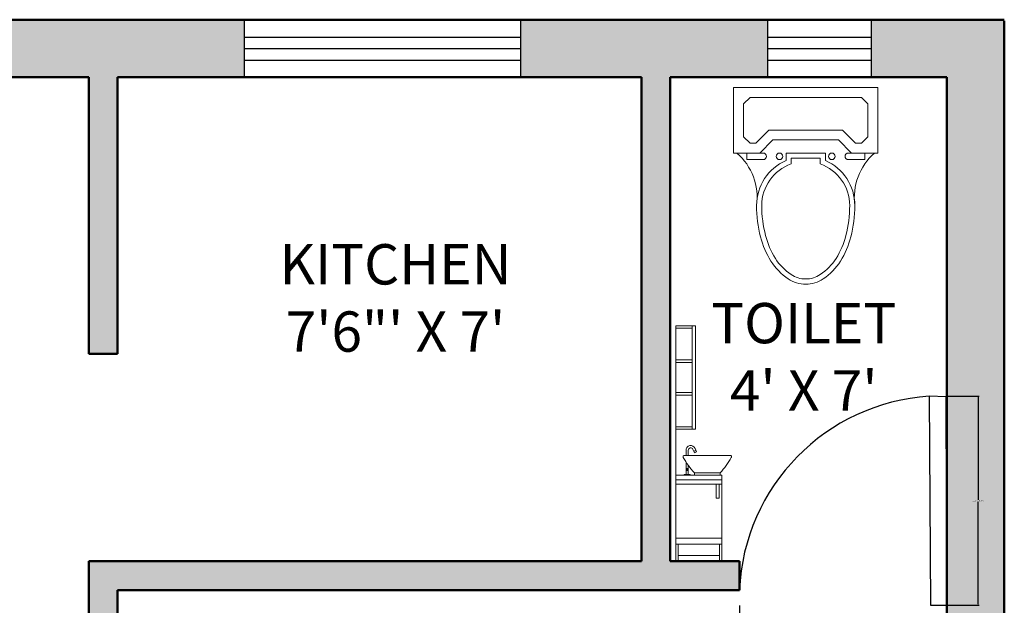
# Model space of a CAD drawing. Units: inches. Extents: x 1771 to 3025, y 319 to 889.
# Tile 35 of 35: x 2854 to 3025, y 788 to 889. Entities that reach past the tile are written whole.
import ezdxf

# ---------------------------------------------------------------- set-up
doc = ezdxf.new("R2010")
doc.units = ezdxf.units.IN
doc.header["$MEASUREMENT"] = 0
for name, color, linetype, lineweight in [('A-ANNO-DIMS', 2, 'Continuous', 18), ('A-AREA-IDEN', 241, 'Continuous', 25), ('A-DOOR', 4, 'Continuous', 25), ('A-FLOR-FIXT', 8, 'Continuous', 18), ('A-GLAZ', 40, 'Continuous', 25), ('A-WALL', 7, 'Continuous', 50), ('A-WALL-PATT', 254, 'Continuous', 13)]:
    doc.layers.add(name, color=color, linetype=linetype, lineweight=lineweight)
doc.styles.get("Standard").update_dxf_attribs({"font": 'arial.ttf'})
doc.dimstyles.get("Standard").update_dxf_attribs({"dimtxt": 0.18, "dimasz": 0.18, "dimexe": 0.18, "dimexo": 0.0625, "dimgap": 0.09, "dimtad": 0, "dimtih": 1, "dimtoh": 1, "dimdec": 4, "dimzin": 0, "dimdsep": 46, "dimtxsty": 'Standard', "dimcen": 0.09, "dimadec": 0, "dimazin": 0, "dimtfac": 1, "dimtdec": 4, "dimtofl": 0, "dimtmove": 0, "dimatfit": 3, "dimfxl": 1, "dimtolj": 1, "dimtzin": 0, "dimarcsym": 0})

# ---------------------------------------------------------------- blocks, each defined once
blk = doc.blocks.new('A$C098B081F')
for p, q in [((558.8, 762), (0, 762)), ((0, 762), (0, 508)), ((558.8, 762), (558.8, 508)), ((63.5, 723.9), (38.1, 698.5)), ((38.1, 698.5), (38.1, 571.5)), ((495.3, 723.9), (63.5, 723.9)), ((520.7, 698.5), (495.3, 723.9)), ((520.7, 698.5), (520.7, 571.5)), ((136.6, 596.9), (85.8, 546.1)), ((422.2, 596.9), (136.6, 596.9)), ((422.2, 596.9), (473, 546.1)), ((38.1, 571.5), (63.5, 546.1)), ((63.5, 546.1), (85.8, 546.1)), ((152.4, 558.8), (101.6, 508)), ((406.4, 558.8), (152.4, 558.8)), ((406.4, 558.8), (457.2, 508)), ((495.3, 546.1), (473, 546.1)), ((495.3, 546.1), (520.7, 571.5)), ((0, 508), (12.7, 508)), ((12.7, 508), (101.6, 508)), ((50.8, 508), (50.8, 482.6)), ((50.8, 508), (101.6, 508)), ((114.3, 508), (101.6, 508)), ((203.2, 508), (203.2, 479.4)), ((203.2, 508), (355.6, 508)), ((355.6, 508), (355.6, 479.4)), ((444.5, 508), (457.2, 508)), ((508, 508), (457.2, 508)), ((508, 508), (546.1, 508)), ((508, 508), (508, 482.6)), ((558.8, 508), (546.1, 508)), ((50.8, 482.6), (114.3, 482.6)), ((223.2, 488), (223.2, 465.8)), ((223.2, 488), (335.6, 488)), ((335.6, 488), (335.6, 465.8)), ((508, 482.6), (444.5, 482.6))]:
    blk.add_line(p, q)
for centre in [(177.8, 495.3), (381, 495.3)]:
    blk.add_circle(centre, 12.7)
for centre, radius, start, end in [((-137.5, 335.8), 228.5, 352.2011, 48.911), ((114.3, 495.3), 12.7, 270, 90), ((444.5, 495.3), 12.7, 90, 270), ((696.3, 335.8), 228.5, 131.089, 187.7989), ((279.4, 304.8), 190.5, 113.5782, 180), ((279.4, 304.8), 170.5, 109.2456, 180), ((279.4, 304.8), 170.5, 0, 70.7544), ((279.4, 304.8), 190.5, 0, 66.4218), ((574.9, 304.8), 486, 180, 194.5143), ((574.9, 304.8), 466, 180, 194.5143), ((-16.1, 304.8), 466, 345.4857, 360), ((-16.1, 304.8), 486, 345.4857, 360), ((429.2, 267.1), 335.5, 194.5143, 212.0054), ((429.2, 267.1), 315.5, 194.5143, 212.0054), ((129.6, 267.1), 315.5, 327.9946, 345.4857), ((129.6, 267.1), 335.5, 327.9946, 345.4857), ((337.2, 209.6), 227, 212.0054, 236.4659), ((337.2, 209.6), 207, 212.0054, 236.4659), ((221.6, 209.6), 207, 303.5341, 327.9946), ((221.6, 209.6), 227, 303.5341, 327.9946), ((279.4, 122.4), 122.4, 236.4659, 270), ((279.4, 122.4), 102.4, 236.4659, 270), ((279.4, 122.4), 102.4, 270, 303.5341), ((279.4, 122.4), 122.4, 270, 303.5341)]:
    blk.add_arc(centre, radius, start, end)
blk = doc.blocks.new('A$C3EAC730C')
for p, q in [((0, 2.05), (0.17, 2.05)), ((0, 2.05), (0, 0.2)), ((0, 2.03), (0.14, 2.03)), ((0.14, 2.05), (0.14, 1.15)), ((0.17, 2.05), (0.17, 1.15)), ((0, 1.7542), (0.14, 1.7542)), ((0, 1.7292), (0.14, 1.7292)), ((0, 1.4708), (0.14, 1.4708)), ((0, 1.4458), (0.14, 1.4458)), ((0, 1.17), (0.14, 1.17)), ((0, 1.15), (0.17, 1.15)), ((0.0877, 0.964), (0.0877, 0.92)), ((0.1077, 0.9647), (0.1077, 0.92)), ((0.1601, 0.9446), (0.1481, 0.9744)), ((0.1545, 0.9582), (0.1731, 0.9657)), ((0.1552, 0.9563), (0.1739, 0.9639)), ((0.1601, 0.9446), (0.1787, 0.9521)), ((0.1787, 0.9521), (0.1666, 0.9819)), ((0.0627, 0.915), (0.0627, 0.9063)), ((0.0677, 0.92), (0.4777, 0.92)), ((0.0877, 0.8637), (0.0877, 0.756)), ((0.4827, 0.915), (0.4827, 0.9063)), ((0.4827, 0.915), (0.4827, 0.9063)), ((0.0902, 0.7905), (0.1052, 0.7905)), ((0.0902, 0.7905), (0.0902, 0.756)), ((0.0947, 0.8022), (0.0947, 0.7905)), ((0.1007, 0.8022), (0.1007, 0.7905)), ((0.1052, 0.7905), (0.1052, 0.756)), ((0.1077, 0.8346), (0.1077, 0.756)), ((0.4, 0.75), (0, 0.75)), ((0.4, 0.71), (0, 0.71)), ((0.0577, 0.75), (0.1037, 0.75)), ((0.0727, 0.756), (0.0727, 0.75)), ((0.1227, 0.756), (0.0727, 0.756)), ((0.1227, 0.756), (0.1227, 0.75)), ((0.1602, 0.77), (0.1602, 0.75)), ((0.1602, 0.77), (0.3852, 0.77)), ((0.1602, 0.75), (0.3852, 0.75)), ((0.3852, 0.77), (0.3852, 0.75)), ((0.4, 0.71), (0.4, 0.75)), ((0.4, 0.72), (0.4, 0.2)), ((0.4, 0.67), (0, 0.67)), ((0.35, 0.55), (0.35, 0.67)), ((0.375, 0.55), (0.375, 0.67)), ((0.35, 0.55), (0.375, 0.55)), ((0.4, 0.2), (0, 0.2)), ((0, 0.2), (0, 0)), ((0.4, 0), (0.4, 0.2)), ((0.4, 0.15), (0, 0.15)), ((0.02, 0.15), (0.02, 0)), ((0.38, 0), (0.38, 0.15)), ((0, 0), (0.4, 0)), ((0.02, 0.05), (0.38, 0.05))]:
    blk.add_line(p, q)
blk.add_circle((0.0977, 0.804), 0.0035)
for centre, radius, start, end in [((0.1286, 0.9665), 0.041, 22.01327, 183.41193), ((0.1286, 0.9665), 0.021, 22.01327, 184.76808), ((0.0677, 0.915), 0.005, 90, 180), ((0.0677, 0.9063), 0.005, 180, 209.45502), ((0.7052, 1.2664), 0.7372, 209.45502, 222.32259), ((-0.1599, 1.2664), 0.7372, 317.67741, 330.54498), ((0.4777, 0.915), 0.005, 0, 90), ((0.4777, 0.9063), 0.005, 330.54498, 0)]:
    blk.add_arc(centre, radius, start, end)
blk = doc.blocks.new('DOOR-35')
blk.add_lwpolyline([(35.88, 36.19), (32.96, 36.3), (33.16, 0), (36, 0.05)], close=True)
blk.add_arc((35.23, 1.11), 35.26, 93.6879, 177.4925)
blk = doc.blocks.new('WIN-48')
for p, q in [((0, 0), (0, 10)), ((48, 0), (48, 10)), ((0, 7), (48, 7)), ((0, 5), (48, 5)), ((0, 3), (48, 3))]:
    blk.add_line(p, q)
blk = doc.blocks.new('WIN-18')
for p, q in [((0, 0), (0, 10)), ((18, 0), (18, 10)), ((0, 7), (18, 7)), ((0, 5), (18, 5)), ((0, 3), (18, 3))]:
    blk.add_line(p, q)
blk = doc.blocks.new('*D30')
at = {"layer": 'A-ANNO-DIMS', "color": 0, "lineweight": -2, "transparency": 16777216}
for p, q in [((3014.75, 824.13), (3020.31, 824.13)), ((3020.13, 823.95), (3020.13, 806.16)), ((3020.13, 788.01), (3020.13, 805.8)), ((3014.75, 787.83), (3020.31, 787.83))]:
    blk.add_line(p, q, dxfattribs=at)
at = {"layer": 'A-ANNO-DIMS', "color": 0, "transparency": 16777216}
for points in [[(3020.1, 823.95), (3020.16, 823.95), (3020.13, 824.13)], [(3020.1, 788.01), (3020.16, 788.01), (3020.13, 787.83)]]:
    blk.add_solid(points, dxfattribs=at)
at = {"layer": 'Defpoints', "color": 0, "transparency": 16777216}
for p in [(3014.68, 824.13), (3020.13, 824.13), (3014.68, 787.83)]:
    blk.add_point(p, dxfattribs=at)
at = {"layer": 'A-ANNO-DIMS', "color": 0, "transparency": 16777216, "insert": (3020.13, 805.98), "char_height": 0.18, "attachment_point": 5}
blk.add_mtext('\\A1;DOOR D2 36 TYP.', dxfattribs=at)
blk = doc.blocks.new('*D31')
at = {"layer": 'A-ANNO-DIMS', "color": 0, "lineweight": -2, "transparency": 16777216}
for p, q in [((2978.68, 787.77), (2978.68, 782.21)), ((3014.68, 787.77), (3014.68, 782.21)), ((2978.86, 782.39), (2996.16, 782.39)), ((3014.5, 782.39), (2997.21, 782.39))]:
    blk.add_line(p, q, dxfattribs=at)
at = {"layer": 'A-ANNO-DIMS', "color": 0, "transparency": 16777216}
for points in [[(2978.86, 782.42), (2978.86, 782.36), (2978.68, 782.39)], [(3014.5, 782.42), (3014.5, 782.36), (3014.68, 782.39)]]:
    blk.add_solid(points, dxfattribs=at)
at = {"layer": 'Defpoints', "color": 0, "transparency": 16777216}
for p in [(2978.68, 787.83), (3014.68, 787.83), (3014.68, 782.39)]:
    blk.add_point(p, dxfattribs=at)
at = {"layer": 'A-ANNO-DIMS', "color": 0, "transparency": 16777216, "insert": (2996.68, 782.39), "char_height": 0.18, "attachment_point": 5}
blk.add_mtext('\\A1;36 TYP.', dxfattribs=at)

msp = doc.modelspace()

# ---------------------------------------------------------------- hatches: boundary and pattern name
at = {"layer": 'A-WALL-PATT'}
h = msp.add_hatch(color=256, dxfattribs=at)
h.dxf.hatch_style = 1
h.paths.add_polyline_path([(2870.68, 879.48), (2892.73, 879.48), (2892.73, 889.48), (2842.68, 889.48), (2842.68, 879.48), (2865.68, 879.48), (2865.68, 831.48), (2870.68, 831.48)])
h.paths.add_polyline_path([(2983.64, 889.48), (2940.73, 889.48), (2940.73, 879.48), (2961.68, 879.48), (2961.68, 795.48), (2865.68, 795.48), (2865.68, 759.48), (2865.68, 665.48), (2870.68, 665.48), (2870.68, 712.85), (2870.68, 790.48), (2978.68, 790.48), (2978.68, 795.48), (2966.68, 795.48), (2966.68, 879.48), (2983.64, 879.48)])
h.paths.add_polyline_path([(3024.68, 889.48), (3001.64, 889.48), (3001.64, 879.48), (3014.68, 879.48), (3014.68, 790.48), (3014.68, 769.46), (3024.68, 769.46)])
h.paths.add_polyline_path([(3024.68, 721.46), (3014.68, 721.46), (3014.68, 670.48), (2906.68, 670.48), (2906.68, 665.48), (2925.68, 665.48), (2925.68, 653.48), (2930.68, 653.48), (2930.68, 665.48), (3014.68, 665.48), (3014.68, 650.02), (3024.68, 650.02)])
h.paths.add_polyline_path([(3024.68, 632.02), (3014.68, 632.02), (3014.68, 617.48), (2925.68, 617.48), (2906.68, 617.48), (2906.68, 612.48), (3014.68, 612.48), (3014.68, 581.96), (3024.68, 581.96)])
h.paths.add_polyline_path([(3024.68, 533.96), (3014.68, 533.96), (3014.68, 480.48), (2870.68, 480.48), (2870.68, 617.48), (2860.68, 617.48), (2860.68, 544.48), (2769.68, 544.48), (2769.68, 534.48), (2860.68, 534.48), (2860.68, 470.48), (3014.68, 470.48), (3014.68, 453.61), (3024.68, 453.61)])
h.paths.add_polyline_path([(3024.68, 405.61), (3014.68, 405.61), (3014.68, 394.48), (2860.68, 394.48), (2860.68, 384.48), (3024.68, 384.48)])
h.paths.add_polyline_path([(2733.68, 643.43), (2723.68, 643.43), (2723.68, 534.48), (2733.68, 534.48)])
h.paths.add_polyline_path([(2733.68, 754.48), (2829.68, 754.48), (2829.68, 759.48), (2733.68, 759.48), (2733.68, 843.44, -0.008336), (2732.38, 843.48), (2723.68, 843.48), (2723.68, 691.43), (2733.68, 691.43)])
h.paths.add_polyline_path([(2794.68, 889.48), (2723.68, 889.48), (2723.68, 879.48), (2794.68, 879.48)])

# ---------------------------------------------------------------- linework, layer by layer
at = {"layer": 'A-WALL'}
for p, q in [((3024.68, 889.48), (2682.68, 889.48)), ((3024.68, 384.48), (3024.68, 889.28)), ((2865.68, 879.48), (2687.68, 879.48)), ((2865.68, 879.48), (2865.68, 831.48)), ((2961.68, 879.48), (2870.68, 879.48)), ((2870.68, 879.48), (2870.68, 831.48)), ((2961.68, 795.48), (2961.68, 879.48)), ((2966.68, 795.48), (2966.68, 879.48)), ((3014.68, 879.48), (2966.68, 879.48)), ((3014.68, 790.48), (3014.68, 879.48)), ((2870.68, 831.48), (2865.68, 831.48)), ((2961.68, 795.48), (2865.68, 795.48)), ((2865.68, 795.48), (2865.68, 759.48)), ((2978.68, 795.48), (2966.68, 795.48)), ((2978.68, 790.48), (2978.68, 795.48)), ((2978.68, 790.48), (2870.68, 790.48)), ((2870.68, 790.48), (2870.68, 670.48)), ((3014.68, 670.48), (3014.68, 790.48))]:
    msp.add_line(p, q, dxfattribs=at)

# ---------------------------------------------------------------- block references
at = {"layer": 'A-DOOR'}
msp.add_blockref('DOOR-35', (2978.68, 787.83), dxfattribs=at)
at = {"layer": 'A-FLOR-FIXT'}
for name, p, xscale, yscale, zscale in [('A$C098B081F', (2977.68, 843.58), 0.0447923195545138, 0.0447923195545138, 0.0447923195545138), ('A$C3EAC730C', (2967.66, 795.48), 19.93356852258053, 19.93356852258053, 19.93356852258053)]:
    msp.add_blockref(name, p, dxfattribs=dict(at, xscale=xscale, yscale=yscale, zscale=zscale))
at = {"layer": 'A-GLAZ'}
for name, p in [('WIN-48', (2892.73, 879.48)), ('WIN-18', (2983.64, 879.48))]:
    msp.add_blockref(name, p, dxfattribs=at)

# ---------------------------------------------------------------- texts
at = {"layer": 'A-AREA-IDEN', "char_height": 7, "attachment_point": 1}
for s, insert in [('\\pxqc;KITCHEN\\P7\'6"\' X 7\'', (2876.22, 850.52)), ("\\pxqc;TOILET\\P4' X 7'", (2947.12, 840.31))]:
    msp.add_mtext_dynamic_manual_height_columns(s, width=85.4611, gutter_width=1, heights=[0], dxfattribs=dict(at, insert=insert))

# ---------------------------------------------------------------- dimensions: what is measured, and where the dimension line sits
at = {"layer": 'A-ANNO-DIMS'}
dim = msp.add_linear_dim(base=(3020.13, 824.13), p1=(3014.68, 787.83), p2=(3014.68, 824.13), angle=90, text='DOOR D2 <> TYP.', dimstyle='Standard', override={"dimdec": 0, "dimrnd": 0, "dimzin": 0, "dimlunit": 2}, dxfattribs=at)
dim.commit()
dim.dimension.update_dxf_attribs({"geometry": '*D30', "text_midpoint": (3020.13, 805.98)})
dim = msp.add_linear_dim(base=(3014.68, 782.39), p1=(2978.68, 787.83), p2=(3014.68, 787.83), text='<> TYP.', dimstyle='Standard', override={"dimdec": 0, "dimrnd": 0, "dimzin": 0, "dimlunit": 2}, dxfattribs=at)
dim.commit()
dim.dimension.update_dxf_attribs({"geometry": '*D31', "text_midpoint": (2996.68, 782.39)})

doc.saveas('drawing.dxf')
